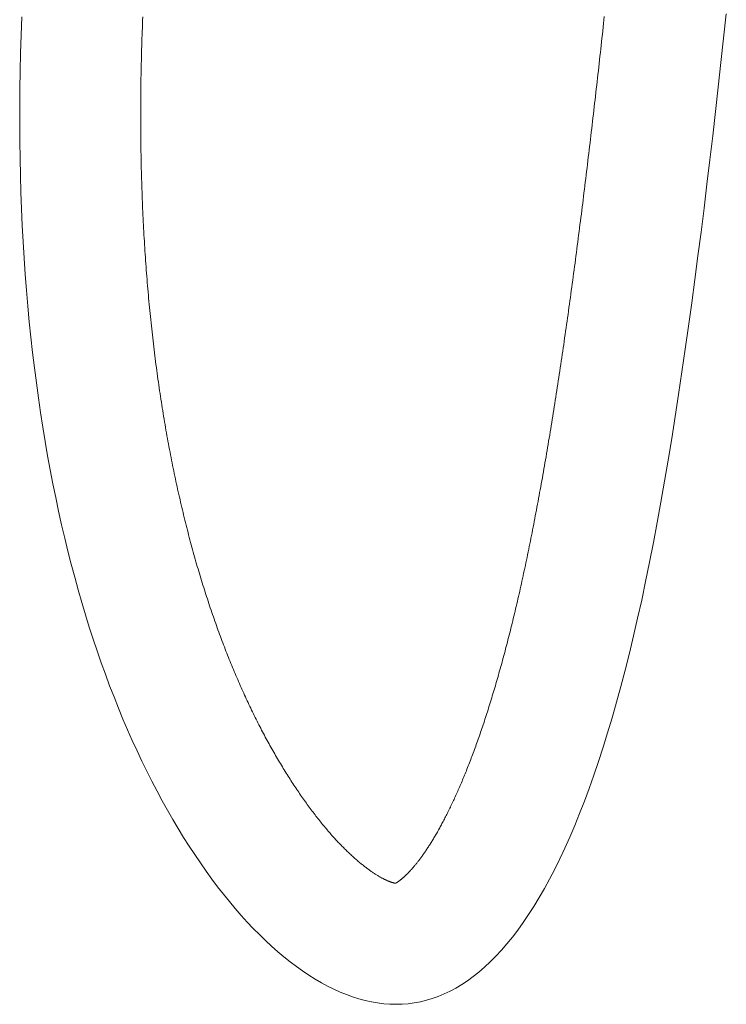
# Model space of a CAD drawing. Units: inches. Extents: x 64 to 1167, y 117 to 939.
# Tile 30 of 56: x 1044.253 to 1048.144, y 442.985 to 448.409. Entities that reach past the tile are written whole.
import ezdxf

# ---------------------------------------------------------------- set-up
doc = ezdxf.new("R2010")
doc.units = ezdxf.units.IN
doc.header["$MEASUREMENT"] = 0
doc.layers.add('A-FLOR-FIXT', color=8, linetype='Continuous', lineweight=18)

# ---------------------------------------------------------------- blocks, each defined once
blk = doc.blocks.new('A$C01277C2D')
for points in [[(2.9158, 4.0746, 0), (2.9049, 3.9738, 0), (2.8939, 3.8729, 0), (2.8827, 3.7721, 0), (2.8713, 3.6713, 0), (2.8597, 3.5708, 0), (2.8479, 3.4705, 0), (2.8359, 3.3706, 0), (2.8237, 3.2711, 0), (2.8114, 3.1721, 0), (2.7988, 3.0738, 0), (2.786, 2.9761, 0), (2.773, 2.8792, 0), (2.7598, 2.7832, 0), (2.7463, 2.6881, 0), (2.7327, 2.5941, 0), (2.7188, 2.5011, 0), (2.7046, 2.4094, 0), (2.6902, 2.3189, 0), (2.6756, 2.2298, 0), (2.6608, 2.1421, 0), (2.6456, 2.056, 0), (2.6303, 1.9715, 0), (2.6146, 1.8887, 0), (2.5987, 1.8077, 0), (2.5825, 1.7285, 0), (2.5661, 1.6513, 0), (2.5494, 1.576, 0), (2.5324, 1.5027, 0), (2.5152, 1.4312, 0), (2.4977, 1.3617, 0), (2.4799, 1.2941, 0), (2.4619, 1.2284, 0), (2.4437, 1.1645, 0), (2.4252, 1.1025, 0), (2.4065, 1.0423, 0), (2.3875, 0.9839, 0), (2.3683, 0.9274, 0), (2.3488, 0.8726, 0), (2.3292, 0.8197, 0), (2.3093, 0.7685, 0), (2.2892, 0.719, 0), (2.2689, 0.6713, 0), (2.2483, 0.6253, 0), (2.2276, 0.5811, 0), (2.2066, 0.5385, 0), (2.1855, 0.4976, 0), (2.1641, 0.4584, 0), (2.1426, 0.4208, 0), (2.1208, 0.3849, 0), (2.0989, 0.3506, 0), (2.0768, 0.318, 0), (2.0545, 0.2869, 0), (2.032, 0.2574, 0), (2.0094, 0.2295, 0), (1.9866, 0.2032, 0), (1.9636, 0.1784, 0), (1.9405, 0.1551, 0), (1.9172, 0.1334, 0), (1.8937, 0.1131, 0), (1.8701, 0.0944, 0), (1.8463, 0.0771, 0), (1.8224, 0.0613, 0), (1.7984, 0.0469, 0), (1.7742, 0.034, 0), (1.7499, 0.0225, 0), (1.7255, 0.0124, 0), (1.7009, 0.0036, 0), (1.6762, -0.0037, 0), (1.6514, -0.0097, 0), (1.6264, -0.0143, 0), (1.6014, -0.0175, 0), (1.5762, -0.0195, 0), (1.551, -0.0201, 0), (1.5256, -0.0195, 0), (1.5002, -0.0175, 0), (1.4746, -0.0143, 0), (1.449, -0.0099, 0), (1.4233, -0.0042, 0), (1.3975, 0.0027, 0), (1.3717, 0.0109, 0), (1.3459, 0.0202, 0), (1.32, 0.0307, 0), (1.2942, 0.0424, 0), (1.2683, 0.0552, 0), (1.2424, 0.0691, 0), (1.2166, 0.0842, 0), (1.1907, 0.1004, 0), (1.1649, 0.1177, 0), (1.1392, 0.136, 0), (1.1135, 0.1554, 0), (1.0879, 0.1759, 0), (1.0623, 0.1974, 0), (1.0369, 0.2199, 0), (1.0115, 0.2434, 0), (0.9863, 0.2679, 0), (0.9612, 0.2934, 0), (0.9362, 0.3198, 0), (0.9114, 0.3472, 0), (0.8867, 0.3755, 0), (0.8622, 0.4047, 0), (0.8378, 0.4349, 0), (0.8137, 0.4659, 0), (0.7897, 0.4978, 0), (0.766, 0.5305, 0), (0.7424, 0.5641, 0), (0.7191, 0.5985, 0), (0.696, 0.6337, 0), (0.6732, 0.6698, 0), (0.6507, 0.7066, 0), (0.6284, 0.7442, 0), (0.6064, 0.7825, 0), (0.5846, 0.8216, 0), (0.5632, 0.8614, 0), (0.5421, 0.9019, 0), (0.5213, 0.9431, 0), (0.5009, 0.985, 0), (0.4808, 1.0275, 0), (0.461, 1.0708, 0), (0.4416, 1.1147, 0), (0.4225, 1.1592, 0), (0.4038, 1.2045, 0), (0.3855, 1.2504, 0), (0.3675, 1.297, 0), (0.3499, 1.3442, 0), (0.3327, 1.3921, 0), (0.3158, 1.4406, 0), (0.2994, 1.4899, 0), (0.2833, 1.5397, 0), (0.2676, 1.5903, 0), (0.2523, 1.6415, 0), (0.2374, 1.6933, 0), (0.2229, 1.7458, 0), (0.2088, 1.799, 0), (0.1951, 1.8528, 0), (0.1819, 1.9073, 0), (0.169, 1.9624, 0), (0.1566, 2.0182, 0), (0.1446, 2.0746, 0), (0.133, 2.1316, 0), (0.1219, 2.1893, 0), (0.1112, 2.2477, 0), (0.101, 2.3067, 0), (0.0912, 2.3663, 0), (0.0818, 2.4266, 0), (0.073, 2.4875, 0), (0.0645, 2.549, 0), (0.0566, 2.6112, 0), (0.0491, 2.674, 0), (0.0421, 2.7375, 0), (0.0355, 2.8016, 0), (0.0295, 2.8663, 0), (0.0239, 2.9316, 0), (0.0188, 2.9976, 0), (0.0142, 3.0642, 0), (0.0101, 3.1315, 0), (0.0065, 3.1993, 0), (0.0034, 3.2678, 0), (0.0008, 3.3369, 0), (-0.0012, 3.4066, 0), (-0.0028, 3.477, 0), (-0.0038, 3.5479, 0), (-0.0043, 3.6195, 0), (-0.0043, 3.6917, 0), (-0.0037, 3.7645, 0), (-0.0026, 3.838, 0), (-0.001, 3.912, 0), (0.0012, 3.9867, 0), (0.004, 4.0619, 0)], [(1.5486, 0.4802, 0), (1.5481, 0.4802, 0), (1.5476, 0.4803, 0), (1.547, 0.4804, 0), (1.5463, 0.4806, 0), (1.5457, 0.4807, 0), (1.545, 0.4809, 0), (1.5442, 0.481, 0), (1.5434, 0.4812, 0), (1.5425, 0.4814, 0), (1.5416, 0.4817, 0), (1.5406, 0.4819, 0), (1.5396, 0.4822, 0), (1.5385, 0.4825, 0), (1.5374, 0.4828, 0), (1.5363, 0.4832, 0), (1.5351, 0.4836, 0), (1.5338, 0.484, 0), (1.5326, 0.4844, 0), (1.5312, 0.4848, 0), (1.5298, 0.4853, 0), (1.5284, 0.4858, 0), (1.5269, 0.4864, 0), (1.5254, 0.4869, 0), (1.5239, 0.4875, 0), (1.5223, 0.4882, 0), (1.5206, 0.4888, 0), (1.5189, 0.4895, 0), (1.5172, 0.4903, 0), (1.5154, 0.491, 0), (1.5136, 0.4918, 0), (1.5117, 0.4927, 0), (1.5098, 0.4935, 0), (1.5078, 0.4945, 0), (1.5058, 0.4954, 0), (1.5038, 0.4964, 0), (1.5017, 0.4974, 0), (1.4995, 0.4985, 0), (1.4974, 0.4996, 0), (1.4951, 0.5008, 0), (1.4929, 0.502, 0), (1.4906, 0.5032, 0), (1.4883, 0.5045, 0), (1.4859, 0.5059, 0), (1.4834, 0.5072, 0), (1.481, 0.5087, 0), (1.4785, 0.5102, 0), (1.4759, 0.5117, 0), (1.4733, 0.5132, 0), (1.4707, 0.5149, 0), (1.468, 0.5165, 0), (1.4653, 0.5183, 0), (1.4626, 0.52, 0), (1.4599, 0.5218, 0), (1.4571, 0.5237, 0), (1.4542, 0.5256, 0), (1.4514, 0.5275, 0), (1.4485, 0.5295, 0), (1.4456, 0.5316, 0), (1.4426, 0.5337, 0), (1.4396, 0.5358, 0), (1.4366, 0.538, 0), (1.4336, 0.5403, 0), (1.4305, 0.5426, 0), (1.4274, 0.5449, 0), (1.4243, 0.5473, 0), (1.4211, 0.5497, 0), (1.4179, 0.5522, 0), (1.4147, 0.5547, 0), (1.4115, 0.5573, 0), (1.4082, 0.5599, 0), (1.4049, 0.5626, 0), (1.4016, 0.5653, 0), (1.3983, 0.5681, 0), (1.3949, 0.5709, 0), (1.3916, 0.5738, 0), (1.3882, 0.5767, 0), (1.3847, 0.5797, 0), (1.3813, 0.5827, 0), (1.3778, 0.5858, 0), (1.3744, 0.5889, 0), (1.3708, 0.5921, 0), (1.3673, 0.5953, 0), (1.3638, 0.5986, 0), (1.3602, 0.6019, 0), (1.3566, 0.6052, 0), (1.3531, 0.6086, 0), (1.3494, 0.6121, 0), (1.3458, 0.6156, 0), (1.3422, 0.6192, 0), (1.3385, 0.6228, 0), (1.3348, 0.6264, 0), (1.3312, 0.6302, 0), (1.3275, 0.6339, 0), (1.3237, 0.6377, 0), (1.32, 0.6416, 0), (1.3163, 0.6455, 0), (1.3125, 0.6494, 0), (1.3088, 0.6534, 0), (1.305, 0.6575, 0), (1.3013, 0.6616, 0), (1.2975, 0.6657, 0), (1.2937, 0.6699, 0), (1.2899, 0.6742, 0), (1.286, 0.6784, 0), (1.2822, 0.6828, 0), (1.2784, 0.6872, 0), (1.2745, 0.6916, 0), (1.2707, 0.6961, 0), (1.2668, 0.7006, 0), (1.263, 0.7051, 0), (1.2591, 0.7097, 0), (1.2552, 0.7144, 0), (1.2513, 0.7191, 0), (1.2474, 0.7239, 0), (1.2435, 0.7286, 0), (1.2396, 0.7335, 0), (1.2357, 0.7384, 0), (1.2318, 0.7433, 0), (1.2279, 0.7483, 0), (1.2239, 0.7533, 0), (1.22, 0.7583, 0), (1.2161, 0.7634, 0), (1.2121, 0.7686, 0), (1.2082, 0.7738, 0), (1.2042, 0.779, 0), (1.2003, 0.7843, 0), (1.1963, 0.7896, 0), (1.1924, 0.795, 0), (1.1884, 0.8004, 0), (1.1844, 0.8058, 0), (1.1804, 0.8113, 0), (1.1765, 0.8168, 0), (1.1725, 0.8224, 0), (1.1685, 0.828, 0), (1.1645, 0.8337, 0), (1.1606, 0.8394, 0), (1.1566, 0.8451, 0), (1.1526, 0.8509, 0), (1.1486, 0.8567, 0), (1.1446, 0.8626, 0), (1.1406, 0.8685, 0), (1.1367, 0.8744, 0), (1.1327, 0.8804, 0), (1.1287, 0.8864, 0), (1.1247, 0.8925, 0), (1.1207, 0.8986, 0), (1.1168, 0.9047, 0), (1.1128, 0.9109, 0), (1.1088, 0.9171, 0), (1.1048, 0.9234, 0), (1.1009, 0.9297, 0), (1.0969, 0.936, 0), (1.0929, 0.9424, 0), (1.089, 0.9488, 0), (1.085, 0.9553, 0), (1.0811, 0.9618, 0), (1.0771, 0.9683, 0), (1.0732, 0.9749, 0), (1.0692, 0.9815, 0), (1.0653, 0.9881, 0), (1.0614, 0.9948, 0), (1.0574, 1.0015, 0), (1.0535, 1.0082, 0), (1.0496, 1.015, 0), (1.0457, 1.0218, 0), (1.0418, 1.0287, 0), (1.0379, 1.0356, 0), (1.034, 1.0425, 0), (1.0301, 1.0495, 0), (1.0262, 1.0565, 0), (1.0224, 1.0635, 0), (1.0185, 1.0706, 0), (1.0146, 1.0777, 0), (1.0108, 1.0848, 0), (1.0069, 1.092, 0), (1.0031, 1.0992, 0), (0.9993, 1.1065, 0), (0.9955, 1.1138, 0), (0.9917, 1.1211, 0), (0.9879, 1.1284, 0), (0.9841, 1.1358, 0), (0.9803, 1.1432, 0), (0.9766, 1.1506, 0), (0.9728, 1.1581, 0), (0.9691, 1.1656, 0), (0.9653, 1.1732, 0), (0.9616, 1.1807, 0), (0.9579, 1.1884, 0), (0.9542, 1.196, 0), (0.9505, 1.2037, 0), (0.9468, 1.2114, 0), (0.9432, 1.2191, 0), (0.9395, 1.2269, 0), (0.9359, 1.2347, 0), (0.9322, 1.2425, 0), (0.9286, 1.2504, 0), (0.925, 1.2583, 0), (0.9214, 1.2662, 0), (0.9178, 1.2741, 0), (0.9142, 1.2821, 0), (0.9106, 1.2902, 0), (0.9071, 1.2982, 0), (0.9035, 1.3063, 0), (0.9, 1.3144, 0), (0.8965, 1.3226, 0), (0.8929, 1.3308, 0), (0.8894, 1.339, 0), (0.8859, 1.3472, 0), (0.8824, 1.3555, 0), (0.879, 1.3638, 0), (0.8755, 1.3721, 0), (0.8721, 1.3805, 0), (0.8686, 1.3889, 0), (0.8652, 1.3974, 0), (0.8618, 1.4058, 0), (0.8584, 1.4143, 0), (0.855, 1.4229, 0), (0.8516, 1.4314, 0), (0.8482, 1.44, 0), (0.8449, 1.4486, 0), (0.8415, 1.4573, 0), (0.8382, 1.466, 0), (0.8349, 1.4747, 0), (0.8316, 1.4835, 0), (0.8283, 1.4923, 0), (0.825, 1.5011, 0), (0.8217, 1.5099, 0), (0.8185, 1.5188, 0), (0.8152, 1.5277, 0), (0.812, 1.5367, 0), (0.8088, 1.5456, 0), (0.8056, 1.5547, 0), (0.8024, 1.5637, 0), (0.7992, 1.5728, 0), (0.7961, 1.5819, 0), (0.7929, 1.591, 0), (0.7898, 1.6002, 0), (0.7866, 1.6094, 0), (0.7835, 1.6186, 0), (0.7804, 1.6278, 0), (0.7773, 1.6371, 0), (0.7743, 1.6464, 0), (0.7712, 1.6558, 0), (0.7682, 1.6652, 0), (0.7651, 1.6746, 0), (0.7621, 1.6841, 0), (0.7591, 1.6935, 0), (0.7561, 1.703, 0), (0.7531, 1.7126, 0), (0.7502, 1.7222, 0), (0.7472, 1.7318, 0), (0.7443, 1.7414, 0), (0.7414, 1.7511, 0), (0.7385, 1.7608, 0), (0.7356, 1.7705, 0), (0.7327, 1.7803, 0), (0.7298, 1.79, 0), (0.727, 1.7999, 0), (0.7241, 1.8097, 0), (0.7213, 1.8196, 0), (0.7185, 1.8295, 0), (0.7157, 1.8395, 0), (0.7129, 1.8495, 0), (0.7102, 1.8595, 0), (0.7074, 1.8695, 0), (0.7047, 1.8796, 0), (0.702, 1.8897, 0), (0.6993, 1.8998, 0), (0.6966, 1.91, 0), (0.6939, 1.9202, 0), (0.6913, 1.9304, 0), (0.6886, 1.9407, 0), (0.686, 1.951, 0), (0.6834, 1.9613, 0), (0.6808, 1.9716, 0), (0.6782, 1.982, 0), (0.6757, 1.9924, 0), (0.6731, 2.0029, 0), (0.6706, 2.0134, 0), (0.6681, 2.0239, 0), (0.6656, 2.0344, 0), (0.6631, 2.045, 0), (0.6606, 2.0556, 0), (0.6582, 2.0662, 0), (0.6558, 2.0769, 0), (0.6533, 2.0876, 0), (0.6509, 2.0983, 0), (0.6485, 2.1091, 0), (0.6462, 2.1199, 0), (0.6438, 2.1307, 0), (0.6415, 2.1415, 0), (0.6392, 2.1524, 0), (0.6369, 2.1633, 0), (0.6346, 2.1742, 0), (0.6323, 2.1852, 0), (0.6301, 2.1962, 0), (0.6278, 2.2073, 0), (0.6256, 2.2183, 0), (0.6234, 2.2294, 0), (0.6212, 2.2405, 0), (0.619, 2.2517, 0), (0.6169, 2.2629, 0), (0.6148, 2.2741, 0), (0.6126, 2.2853, 0), (0.6105, 2.2966, 0), (0.6085, 2.3079, 0), (0.6064, 2.3193, 0), (0.6043, 2.3306, 0), (0.6023, 2.342, 0), (0.6003, 2.3535, 0), (0.5983, 2.3649, 0), (0.5963, 2.3764, 0), (0.5944, 2.388, 0), (0.5924, 2.3995, 0), (0.5905, 2.4111, 0), (0.5886, 2.4227, 0), (0.5867, 2.4343, 0), (0.5848, 2.446, 0), (0.583, 2.4577, 0), (0.5811, 2.4695, 0), (0.5793, 2.4812, 0), (0.5775, 2.493, 0), (0.5757, 2.5048, 0), (0.574, 2.5167, 0), (0.5722, 2.5286, 0), (0.5705, 2.5405, 0), (0.5688, 2.5524, 0), (0.5671, 2.5644, 0), (0.5654, 2.5764, 0), (0.5637, 2.5885, 0), (0.5621, 2.6005, 0), (0.5605, 2.6126, 0), (0.5589, 2.6248, 0), (0.5573, 2.6369, 0), (0.5558, 2.6491, 0), (0.5542, 2.6613, 0), (0.5527, 2.6736, 0), (0.5512, 2.6858, 0), (0.5497, 2.6982, 0), (0.5482, 2.7105, 0), (0.5468, 2.7229, 0), (0.5453, 2.7353, 0), (0.5439, 2.7477, 0), (0.5425, 2.7601, 0), (0.5412, 2.7726, 0), (0.5398, 2.7851, 0), (0.5385, 2.7977, 0), (0.5372, 2.8103, 0), (0.5359, 2.8229, 0), (0.5346, 2.8355, 0), (0.5334, 2.8482, 0), (0.5321, 2.8609, 0), (0.5309, 2.8736, 0), (0.5297, 2.8864, 0), (0.5285, 2.8992, 0), (0.5274, 2.912, 0), (0.5262, 2.9248, 0), (0.5251, 2.9377, 0), (0.524, 2.9506, 0), (0.5229, 2.9635, 0), (0.5219, 2.9765, 0), (0.5208, 2.9895, 0), (0.5198, 3.0025, 0), (0.5188, 3.0156, 0), (0.5179, 3.0286, 0), (0.5169, 3.0418, 0), (0.516, 3.0549, 0), (0.5151, 3.0681, 0), (0.5142, 3.0813, 0), (0.5133, 3.0945, 0), (0.5124, 3.1078, 0), (0.5116, 3.1211, 0), (0.5108, 3.1344, 0), (0.51, 3.1477, 0), (0.5092, 3.1611, 0), (0.5085, 3.1745, 0), (0.5078, 3.188, 0), (0.5071, 3.2014, 0), (0.5064, 3.2149, 0), (0.5057, 3.2285, 0), (0.5051, 3.242, 0), (0.5044, 3.2556, 0), (0.5038, 3.2692, 0), (0.5033, 3.2829, 0), (0.5027, 3.2966, 0), (0.5022, 3.3103, 0), (0.5016, 3.324, 0), (0.5012, 3.3378, 0), (0.5007, 3.3516, 0), (0.5002, 3.3654, 0), (0.4998, 3.3792, 0), (0.4994, 3.3931, 0), (0.499, 3.407, 0), (0.4986, 3.421, 0), (0.4983, 3.435, 0), (0.498, 3.4489, 0), (0.4977, 3.463, 0), (0.4974, 3.477, 0), (0.4971, 3.4911, 0), (0.4969, 3.5052, 0), (0.4967, 3.5194, 0), (0.4965, 3.5335, 0), (0.4963, 3.5478, 0), (0.4962, 3.562, 0), (0.496, 3.5762, 0), (0.4959, 3.5905, 0), (0.4959, 3.6048, 0), (0.4958, 3.6192, 0), (0.4958, 3.6336, 0), (0.4958, 3.648, 0), (0.4958, 3.6624, 0), (0.4958, 3.6769, 0), (0.4958, 3.6913, 0), (0.4959, 3.7059, 0), (0.496, 3.7204, 0), (0.4961, 3.735, 0), (0.4963, 3.7496, 0), (0.4964, 3.7642, 0), (0.4966, 3.7789, 0), (0.4968, 3.7936, 0), (0.497, 3.8083, 0), (0.4973, 3.823, 0), (0.4976, 3.8378, 0), (0.4979, 3.8526, 0), (0.4982, 3.8674, 0), (0.4985, 3.8823, 0), (0.4989, 3.8972, 0), (0.4993, 3.9121, 0), (0.4997, 3.927, 0), (0.5001, 3.942, 0), (0.5006, 3.957, 0), (0.5011, 3.972, 0), (0.5016, 3.987, 0), (0.5021, 4.0021, 0), (0.5026, 4.0172, 0), (0.5032, 4.0324, 0), (0.5038, 4.0475, 0), (0.5044, 4.0627, 0)], [(2.4117, 4.064, 0), (2.4101, 4.049, 0), (2.4085, 4.034, 0), (2.4068, 4.019, 0), (2.4052, 4.004, 0), (2.4036, 3.989, 0), (2.4019, 3.974, 0), (2.4003, 3.959, 0), (2.3986, 3.9441, 0), (2.397, 3.9291, 0), (2.3953, 3.9141, 0), (2.3937, 3.8991, 0), (2.392, 3.8841, 0), (2.3903, 3.8692, 0), (2.3887, 3.8542, 0), (2.387, 3.8392, 0), (2.3853, 3.8243, 0), (2.3836, 3.8093, 0), (2.3819, 3.7944, 0), (2.3803, 3.7794, 0), (2.3786, 3.7645, 0), (2.3769, 3.7495, 0), (2.3752, 3.7346, 0), (2.3735, 3.7197, 0), (2.3718, 3.7047, 0), (2.37, 3.6898, 0), (2.3683, 3.6749, 0), (2.3666, 3.66, 0), (2.3649, 3.6451, 0), (2.3631, 3.6302, 0), (2.3614, 3.6154, 0), (2.3597, 3.6005, 0), (2.3579, 3.5856, 0), (2.3562, 3.5708, 0), (2.3544, 3.5559, 0), (2.3527, 3.5411, 0), (2.3509, 3.5263, 0), (2.3492, 3.5115, 0), (2.3474, 3.4967, 0), (2.3456, 3.4819, 0), (2.3439, 3.4671, 0), (2.3421, 3.4523, 0), (2.3403, 3.4376, 0), (2.3385, 3.4228, 0), (2.3367, 3.4081, 0), (2.3349, 3.3933, 0), (2.3331, 3.3786, 0), (2.3313, 3.3639, 0), (2.3295, 3.3493, 0), (2.3277, 3.3346, 0), (2.3259, 3.3199, 0), (2.3241, 3.3053, 0), (2.3223, 3.2907, 0), (2.3204, 3.2761, 0), (2.3186, 3.2614, 0), (2.3168, 3.2469, 0), (2.3149, 3.2323, 0), (2.3131, 3.2178, 0), (2.3112, 3.2032, 0), (2.3094, 3.1887, 0), (2.3075, 3.1742, 0), (2.3057, 3.1597, 0), (2.3038, 3.1452, 0), (2.302, 3.1308, 0), (2.3001, 3.1164, 0), (2.2982, 3.1019, 0), (2.2963, 3.0875, 0), (2.2944, 3.0732, 0), (2.2925, 3.0588, 0), (2.2906, 3.0445, 0), (2.2887, 3.0301, 0), (2.2868, 3.0158, 0), (2.2849, 3.0016, 0), (2.283, 2.9873, 0), (2.2811, 2.9731, 0), (2.2792, 2.9589, 0), (2.2773, 2.9447, 0), (2.2753, 2.9305, 0), (2.2734, 2.9163, 0), (2.2715, 2.9022, 0), (2.2695, 2.8881, 0), (2.2676, 2.874, 0), (2.2656, 2.86, 0), (2.2637, 2.8459, 0), (2.2617, 2.8319, 0), (2.2597, 2.8179, 0), (2.2578, 2.804, 0), (2.2558, 2.79, 0), (2.2538, 2.7761, 0), (2.2518, 2.7622, 0), (2.2498, 2.7484, 0), (2.2478, 2.7345, 0), (2.2458, 2.7207, 0), (2.2438, 2.7069, 0), (2.2418, 2.6932, 0), (2.2398, 2.6794, 0), (2.2378, 2.6657, 0), (2.2358, 2.6521, 0), (2.2338, 2.6384, 0), (2.2317, 2.6248, 0), (2.2297, 2.6112, 0), (2.2277, 2.5976, 0), (2.2256, 2.5841, 0), (2.2236, 2.5706, 0), (2.2215, 2.5571, 0), (2.2195, 2.5437, 0), (2.2174, 2.5303, 0), (2.2153, 2.5169, 0), (2.2133, 2.5035, 0), (2.2112, 2.4902, 0), (2.2091, 2.4769, 0), (2.207, 2.4636, 0), (2.2049, 2.4504, 0), (2.2028, 2.4372, 0), (2.2007, 2.4241, 0), (2.1986, 2.411, 0), (2.1965, 2.3979, 0), (2.1944, 2.3848, 0), (2.1923, 2.3718, 0), (2.1902, 2.3588, 0), (2.188, 2.3459, 0), (2.1859, 2.333, 0), (2.1838, 2.3201, 0), (2.1816, 2.3073, 0), (2.1795, 2.2945, 0), (2.1773, 2.2818, 0), (2.1752, 2.2691, 0), (2.173, 2.2564, 0), (2.1709, 2.2437, 0), (2.1687, 2.2311, 0), (2.1665, 2.2186, 0), (2.1643, 2.206, 0), (2.1622, 2.1936, 0), (2.16, 2.1811, 0), (2.1578, 2.1687, 0), (2.1556, 2.1564, 0), (2.1534, 2.144, 0), (2.1512, 2.1317, 0), (2.149, 2.1195, 0), (2.1467, 2.1073, 0), (2.1445, 2.0951, 0), (2.1423, 2.083, 0), (2.1401, 2.0709, 0), (2.1379, 2.0589, 0), (2.1356, 2.0469, 0), (2.1334, 2.035, 0), (2.1311, 2.0231, 0), (2.1289, 2.0112, 0), (2.1266, 1.9994, 0), (2.1244, 1.9876, 0), (2.1221, 1.9759, 0), (2.1199, 1.9642, 0), (2.1176, 1.9525, 0), (2.1153, 1.9409, 0), (2.113, 1.9294, 0), (2.1108, 1.9179, 0), (2.1085, 1.9064, 0), (2.1062, 1.895, 0), (2.1039, 1.8836, 0), (2.1016, 1.8723, 0), (2.0993, 1.861, 0), (2.097, 1.8498, 0), (2.0947, 1.8386, 0), (2.0924, 1.8274, 0), (2.09, 1.8163, 0), (2.0877, 1.8053, 0), (2.0854, 1.7943, 0), (2.083, 1.7833, 0), (2.0807, 1.7724, 0), (2.0784, 1.7616, 0), (2.076, 1.7508, 0), (2.0737, 1.74, 0), (2.0713, 1.7293, 0), (2.069, 1.7186, 0), (2.0666, 1.708, 0), (2.0642, 1.6975, 0), (2.0619, 1.6869, 0), (2.0595, 1.6765, 0), (2.0571, 1.6661, 0), (2.0547, 1.6557, 0), (2.0523, 1.6454, 0), (2.0499, 1.6351, 0), (2.0475, 1.6249, 0), (2.0451, 1.6148, 0), (2.0427, 1.6046, 0), (2.0403, 1.5946, 0), (2.0379, 1.5845, 0), (2.0355, 1.5746, 0), (2.0331, 1.5646, 0), (2.0307, 1.5548, 0), (2.0282, 1.5449, 0), (2.0258, 1.5351, 0), (2.0234, 1.5254, 0), (2.0209, 1.5157, 0), (2.0185, 1.506, 0), (2.016, 1.4964, 0), (2.0136, 1.4869, 0), (2.0111, 1.4773, 0), (2.0087, 1.4679, 0), (2.0062, 1.4585, 0), (2.0038, 1.4491, 0), (2.0013, 1.4398, 0), (1.9988, 1.4305, 0), (1.9963, 1.4212, 0), (1.9939, 1.4121, 0), (1.9914, 1.4029, 0), (1.9889, 1.3938, 0), (1.9864, 1.3848, 0), (1.9839, 1.3758, 0), (1.9814, 1.3668, 0), (1.9789, 1.3579, 0), (1.9764, 1.3491, 0), (1.974, 1.3402, 0), (1.9714, 1.3315, 0), (1.9689, 1.3228, 0), (1.9664, 1.3141, 0), (1.9639, 1.3054, 0), (1.9614, 1.2969, 0), (1.9589, 1.2883, 0), (1.9564, 1.2798, 0), (1.9539, 1.2714, 0), (1.9513, 1.263, 0), (1.9488, 1.2547, 0), (1.9463, 1.2464, 0), (1.9438, 1.2381, 0), (1.9412, 1.2299, 0), (1.9387, 1.2217, 0), (1.9362, 1.2136, 0), (1.9337, 1.2055, 0), (1.9311, 1.1975, 0), (1.9286, 1.1895, 0), (1.926, 1.1816, 0), (1.9235, 1.1737, 0), (1.9209, 1.1659, 0), (1.9184, 1.1581, 0), (1.9159, 1.1503, 0), (1.9133, 1.1426, 0), (1.9108, 1.1349, 0), (1.9082, 1.1273, 0), (1.9057, 1.1198, 0), (1.9031, 1.1123, 0), (1.9005, 1.1048, 0), (1.898, 1.0974, 0), (1.8954, 1.09, 0), (1.8929, 1.0826, 0), (1.8903, 1.0754, 0), (1.8878, 1.0681, 0), (1.8852, 1.0609, 0), (1.8826, 1.0538, 0), (1.8801, 1.0467, 0), (1.8775, 1.0396, 0), (1.875, 1.0326, 0), (1.8724, 1.0256, 0), (1.8698, 1.0187, 0), (1.8673, 1.0119, 0), (1.8647, 1.005, 0), (1.8621, 0.9983, 0), (1.8596, 0.9915, 0), (1.857, 0.9848, 0), (1.8544, 0.9782, 0), (1.8518, 0.9716, 0), (1.8493, 0.9651, 0), (1.8467, 0.9586, 0), (1.8441, 0.9521, 0), (1.8416, 0.9457, 0), (1.839, 0.9393, 0), (1.8364, 0.933, 0), (1.8339, 0.9267, 0), (1.8313, 0.9205, 0), (1.8288, 0.9143, 0), (1.8262, 0.9082, 0), (1.8236, 0.9021, 0), (1.8211, 0.8961, 0), (1.8185, 0.8901, 0), (1.816, 0.8841, 0), (1.8134, 0.8782, 0), (1.8109, 0.8724, 0), (1.8083, 0.8666, 0), (1.8058, 0.8608, 0), (1.8032, 0.8551, 0), (1.8007, 0.8494, 0), (1.7981, 0.8438, 0), (1.7956, 0.8382, 0), (1.7931, 0.8327, 0), (1.7906, 0.8272, 0), (1.788, 0.8218, 0), (1.7855, 0.8164, 0), (1.783, 0.811, 0), (1.7805, 0.8057, 0), (1.778, 0.8004, 0), (1.7755, 0.7952, 0), (1.773, 0.7901, 0), (1.7705, 0.7849, 0), (1.768, 0.7799, 0), (1.7655, 0.7748, 0), (1.763, 0.7699, 0), (1.7605, 0.7649, 0), (1.7581, 0.76, 0), (1.7556, 0.7552, 0), (1.7531, 0.7504, 0), (1.7507, 0.7456, 0), (1.7482, 0.7409, 0), (1.7458, 0.7362, 0), (1.7434, 0.7316, 0), (1.7409, 0.727, 0), (1.7385, 0.7225, 0), (1.7361, 0.718, 0), (1.7337, 0.7136, 0), (1.7313, 0.7092, 0), (1.7289, 0.7049, 0), (1.7265, 0.7006, 0), (1.7241, 0.6963, 0), (1.7217, 0.6921, 0), (1.7193, 0.6879, 0), (1.717, 0.6838, 0), (1.7146, 0.6797, 0), (1.7123, 0.6757, 0), (1.7099, 0.6717, 0), (1.7076, 0.6678, 0), (1.7053, 0.6639, 0), (1.703, 0.6601, 0), (1.7006, 0.6563, 0), (1.6984, 0.6525, 0), (1.6961, 0.6488, 0), (1.6938, 0.6451, 0), (1.6915, 0.6415, 0), (1.6892, 0.6379, 0), (1.687, 0.6344, 0), (1.6847, 0.6309, 0), (1.6825, 0.6275, 0), (1.6803, 0.6241, 0), (1.6781, 0.6207, 0), (1.6759, 0.6174, 0), (1.6737, 0.6142, 0), (1.6715, 0.611, 0), (1.6693, 0.6078, 0), (1.6671, 0.6047, 0), (1.665, 0.6016, 0), (1.6629, 0.5986, 0), (1.6607, 0.5956, 0), (1.6586, 0.5927, 0), (1.6565, 0.5898, 0), (1.6544, 0.5869, 0), (1.6524, 0.5841, 0), (1.6503, 0.5814, 0), (1.6483, 0.5787, 0), (1.6463, 0.576, 0), (1.6442, 0.5734, 0), (1.6422, 0.5708, 0), (1.6403, 0.5682, 0), (1.6383, 0.5657, 0), (1.6363, 0.5633, 0), (1.6344, 0.5609, 0), (1.6325, 0.5585, 0), (1.6306, 0.5562, 0), (1.6287, 0.5539, 0), (1.6268, 0.5517, 0), (1.625, 0.5494, 0), (1.6231, 0.5473, 0), (1.6213, 0.5452, 0), (1.6195, 0.5431, 0), (1.6177, 0.541, 0), (1.6159, 0.539, 0), (1.6142, 0.5371, 0), (1.6124, 0.5352, 0), (1.6107, 0.5333, 0), (1.609, 0.5314, 0), (1.6074, 0.5296, 0), (1.6057, 0.5278, 0), (1.6041, 0.5261, 0), (1.6024, 0.5244, 0), (1.6008, 0.5228, 0), (1.5993, 0.5211, 0), (1.5977, 0.5196, 0), (1.5961, 0.518, 0), (1.5946, 0.5165, 0), (1.5931, 0.515, 0), (1.5917, 0.5136, 0), (1.5902, 0.5122, 0), (1.5888, 0.5108, 0), (1.5873, 0.5095, 0), (1.5859, 0.5082, 0), (1.5846, 0.5069, 0), (1.5832, 0.5057, 0), (1.5819, 0.5045, 0), (1.5806, 0.5033, 0), (1.5793, 0.5022, 0), (1.5781, 0.5011, 0), (1.5768, 0.5, 0), (1.5756, 0.499, 0), (1.5744, 0.498, 0), (1.5733, 0.497, 0), (1.5721, 0.4961, 0), (1.571, 0.4952, 0), (1.5699, 0.4943, 0), (1.5689, 0.4935, 0), (1.5678, 0.4927, 0), (1.5668, 0.4919, 0), (1.5658, 0.4911, 0), (1.5648, 0.4904, 0), (1.5639, 0.4897, 0), (1.563, 0.4891, 0), (1.5621, 0.4884, 0), (1.5612, 0.4878, 0), (1.5604, 0.4872, 0), (1.5596, 0.4867, 0), (1.5588, 0.4862, 0), (1.558, 0.4857, 0), (1.5573, 0.4852, 0), (1.5566, 0.4847, 0), (1.5559, 0.4843, 0), (1.5553, 0.4839, 0), (1.5546, 0.4835, 0), (1.554, 0.4831, 0), (1.5534, 0.4828, 0), (1.5529, 0.4825, 0), (1.5523, 0.4822, 0), (1.5518, 0.4819, 0), (1.5513, 0.4816, 0), (1.5509, 0.4813, 0), (1.5504, 0.4811, 0), (1.55, 0.4809, 0), (1.5496, 0.4807, 0), (1.5493, 0.4805, 0), (1.5489, 0.4803, 0), (1.5486, 0.4802, 0)]]:
    blk.add_polyline3d(points)

msp = doc.modelspace()

# ---------------------------------------------------------------- block references
at = {"layer": 'A-FLOR-FIXT', "xscale": 1.33257137012807, "yscale": 1.33257137012807, "zscale": 1.33257137012807}
msp.add_blockref('A$C01277C2D', (1044.2585, 443.012), dxfattribs=at)

doc.saveas('drawing.dxf')
